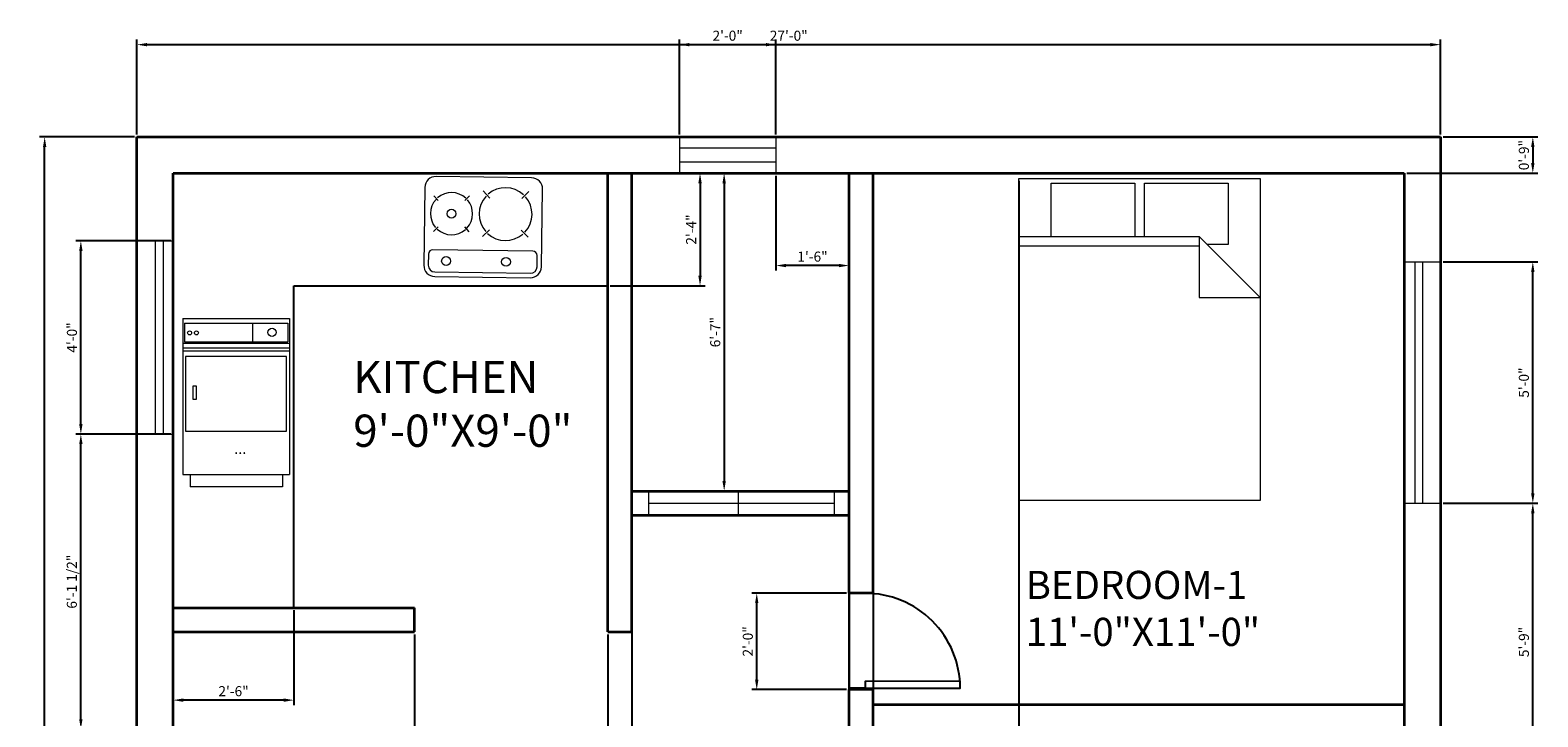
# Model space of a CAD drawing. Units: inches. Extents: x -2945 to -2182, y 3541 to 4172.
# Tile 5 of 5: x -2558 to -2183, y 3865 to 4036. Entities that reach past the tile are written whole.
import ezdxf
from ezdxf.enums import TextEntityAlignment as Align

# ---------------------------------------------------------------- set-up
doc = ezdxf.new("R2010")
doc.units = ezdxf.units.IN
for name, color, linetype, lineweight in [('A-ANNO-DIMS', 2, 'Continuous', 18), ('A-AREA-IDEN', 7, 'Continuous', 18), ('A-DOOR', 3, 'Continuous', 25), ('A-EQPM', 8, 'Continuous', 18), ('A-FLOR-FIXT', 9, 'Continuous', 25), ('A-FURN', 9, 'Continuous', 18), ('A-GLAZ', 4, 'Continuous', 18), ('A-WALL', 7, 'Continuous', 35)]:
    doc.layers.add(name, color=color, linetype=linetype, lineweight=lineweight)
doc.styles.add('OPUS', font='txt')
doc.styles.get("Standard").update_dxf_attribs({"font": 'arial.ttf'})
doc.dimstyles.new('ISO-25', dxfattribs={"dimtxt": 2.5, "dimasz": 2.5, "dimexe": 1.25, "dimexo": 0.625, "dimtad": 1, "dimdec": 0, "dimlunit": 3, "dimtxsty": 'Standard', "dimcen": 2.5, "dimadec": 0, "dimazin": 0, "dimtfac": 1, "dimtdec": 0, "dimtmove": 0, "dimatfit": 3, "dimfxl": 1, "dimarcsym": 0})

# ---------------------------------------------------------------- blocks, each defined once
blk = doc.blocks.new('Bed - Queen')
for p, q in [((0, -80.00003), (0, 0)), ((0, 0), (59.99999, 0)), ((59.99999, 0), (59.99999, -80.00003)), ((7.99999, -1.2), (28.79998, -1.2)), ((7.99999, -14.4), (7.99999, -1.2)), ((28.79998, -1.2), (28.79998, -14.4)), ((31.19999, -1.2), (51.99999, -1.2)), ((31.19999, -14.4), (31.19999, -1.2)), ((51.99999, -1.2), (51.99999, -16.4)), ((0, -14.4), (44.8, -14.4)), ((59.99999, -29.6), (44.8, -14.4)), ((44.8, -14.4), (44.8, -29.6)), ((44.8, -16.8), (0, -16.8)), ((51.99999, -16.4), (46.79936, -16.4)), ((44.8, -29.6), (59.99999, -29.6)), ((59.99999, -80.00003), (0, -80.00003))]:
    blk.add_line(p, q)
blk = doc.blocks.new('*U5')
for p, q in [((-600, 0), (-600, -100)), ((0, 0), (0, -100))]:
    blk.add_line(p, q)
blk.add_lwpolyline([(0, 0), (0, 600), (-43.75, 600), (-43.75, 0)], close=True)
blk.add_arc((0, 0), 600, 90, 180)
blk = doc.blocks.new('COOKTOP-2B')
for p, q in [((26.79, 24.83), (3.07, 25.16)), ((0.27, 22.44), (0, 3.13)), ((2.48, 20.39), (3.6, 19.22)), ((11.35, 20.32), (10.18, 19.2)), ((14.72, 21.57), (16.43, 19.81)), ((26.08, 21.42), (24.32, 19.71)), ((29.25, 2.72), (29.51, 22.03)), ((2.41, 11.52), (3.59, 12.64)), ((11.28, 11.45), (10.16, 12.63)), ((14.56, 10.21), (16.33, 11.92)), ((25.93, 10.06), (24.22, 11.82)), ((1.14, 5.87), (1.1, 3.11)), ((27.09, 6.61), (2.26, 6.96)), ((28.14, 2.74), (28.18, 5.5)), ((2.72, 0.33), (26.45, 0)), ((2.74, 1.43), (26.46, 1.1))]:
    blk.add_line(p, q)
for centre in [(6.88, 15.92), (5.53, 4.15), (20.43, 3.95)]:
    blk.add_circle(centre, 1.1)
for centre, radius, start, end in [((3.03, 22.4), 2.76, 89.203, 179.203), ((26.76, 22.07), 2.76, 359.203, 89.203), ((6.88, 15.92), 5.24, 137.22, 221.186), ((6.88, 15.92), 5.24, 47.22, 131.186), ((6.88, 15.92), 5.24, 317.22, 41.186), ((20.32, 15.81), 6.57, 137.22, 221.186), ((20.32, 15.81), 6.57, 47.22, 131.186), ((20.32, 15.81), 6.57, 317.22, 41.186), ((6.88, 15.92), 5.24, 227.22, 311.186), ((20.32, 15.81), 6.57, 227.22, 311.186), ((2.25, 5.86), 1.1, 89.203, 179.203), ((27.08, 5.51), 1.1, 359.203, 89.203), ((2.76, 3.09), 2.76, 179.203, 269.203), ((2.76, 3.09), 1.66, 179.203, 269.203), ((26.49, 2.76), 2.76, 269.203, 359.203), ((26.49, 2.76), 1.66, 269.203, 359.203)]:
    blk.add_arc(centre, radius, start, end)
blk = doc.blocks.new('KITCHEN-APPLIANCE-FRONT')
for p, q in [((0, 41.84), (0, 3.07)), ((0, 41.84), (26.49, 41.84)), ((26.49, 41.84), (26.49, 3.07)), ((0.38, 40.69), (0.38, 36.08)), ((0.38, 40.69), (26.1, 40.69)), ((17.27, 40.69), (17.27, 36.08)), ((26.1, 40.69), (26.1, 36.08)), ((0, 35.7), (26.49, 35.7)), ((0, 34.55), (26.49, 34.55)), ((0, 33.78), (26.49, 33.78)), ((0.38, 36.08), (26.1, 36.08)), ((0, 3.07), (26.49, 3.07)), ((1.77, 3.07), (1.77, 0)), ((24.72, 0), (1.77, 0)), ((24.72, 3.07), (24.72, 0))]:
    blk.add_line(p, q)
for points in [[(0.62, 13.82), (25.76, 13.82), (25.76, 32.44), (0.62, 32.44)], [(2.53, 21.69), (2.53, 25.14), (3.3, 25.14), (3.3, 21.69)]]:
    blk.add_lwpolyline(points, close=True)
for centre, radius in [((1.65, 38.28), 0.491), ((3.34, 38.28), 0.491), ((22.13, 38.4), 1.02)]:
    blk.add_circle(centre, radius)
at = {"style": 'OPUS'}
blk.add_text('...', height=2.65, dxfattribs=at).set_placement((14.24, 8.2), align=Align.CENTER)
blk = doc.blocks.new('*D20')
at = {"layer": 'A-ANNO-DIMS', "color": 0, "lineweight": -2, "transparency": 16777216}
for p, q in [((-2531.05, 4010.2), (-2531.05, 4033.78)), ((-2528.55, 4032.53), (-2209.55, 4032.53)), ((-2207.05, 4010.2), (-2207.05, 4033.78))]:
    blk.add_line(p, q, dxfattribs=at)
at = {"layer": 'A-ANNO-DIMS', "color": 0, "transparency": 16777216}
for points in [[(-2528.55, 4032.94), (-2528.55, 4032.11), (-2531.05, 4032.53)], [(-2209.55, 4032.94), (-2209.55, 4032.11), (-2207.05, 4032.53)]]:
    blk.add_solid(points, dxfattribs=at)
at = {"layer": 'Defpoints', "color": 0, "transparency": 16777216}
for p in [(-2207.05, 4032.53), (-2531.05, 4009.58), (-2207.05, 4009.58)]:
    blk.add_point(p, dxfattribs=at)
at = {"layer": 'A-ANNO-DIMS', "color": 0, "transparency": 16777216, "insert": (-2369.05, 4034.43), "char_height": 2.5, "attachment_point": 5}
blk.add_mtext('27\'-0"', dxfattribs=at)
blk = doc.blocks.new('*D21')
at = {"layer": 'A-ANNO-DIMS', "color": 0, "lineweight": -2, "transparency": 16777216}
for p, q in [((-2531.67, 4009.58), (-2555.25, 4009.58)), ((-2554, 3568.08), (-2554, 4007.08)), ((-2531.67, 3565.58), (-2555.25, 3565.58))]:
    blk.add_line(p, q, dxfattribs=at)
at = {"layer": 'A-ANNO-DIMS', "color": 0, "transparency": 16777216}
for points in [[(-2554.42, 4007.08), (-2553.58, 4007.08), (-2554, 4009.58)], [(-2554.42, 3568.08), (-2553.58, 3568.08), (-2554, 3565.58)]]:
    blk.add_solid(points, dxfattribs=at)
at = {"layer": 'Defpoints', "color": 0, "transparency": 16777216}
for p in [(-2554, 4009.58), (-2531.05, 4009.58), (-2531.05, 3565.58)]:
    blk.add_point(p, dxfattribs=at)
at = {"layer": 'A-ANNO-DIMS', "color": 0, "transparency": 16777216, "insert": (-2555.9, 3787.58), "char_height": 2.5, "attachment_point": 5, "rotation": 90}
blk.add_mtext('37\'-0"', dxfattribs=at)
blk = doc.blocks.new('*D29')
at = {"layer": 'A-ANNO-DIMS', "color": 0, "lineweight": -2, "transparency": 16777216}
for p, q in [((-2522.67, 3935.75), (-2546.25, 3935.75)), ((-2545, 3864.89), (-2545, 3933.25)), ((-2522.67, 3862.39), (-2546.25, 3862.39))]:
    blk.add_line(p, q, dxfattribs=at)
at = {"layer": 'A-ANNO-DIMS', "color": 0, "transparency": 16777216}
for points in [[(-2545.42, 3933.25), (-2544.58, 3933.25), (-2545, 3935.75)], [(-2545.42, 3864.89), (-2544.58, 3864.89), (-2545, 3862.39)]]:
    blk.add_solid(points, dxfattribs=at)
at = {"layer": 'Defpoints', "color": 0, "transparency": 16777216}
for p in [(-2545, 3935.75), (-2522.05, 3935.75), (-2522.05, 3862.39)]:
    blk.add_point(p, dxfattribs=at)
at = {"layer": 'A-ANNO-DIMS', "color": 0, "transparency": 16777216, "insert": (-2546.92, 3899.07), "char_height": 2.5, "attachment_point": 5, "rotation": 90}
blk.add_mtext('6\'-1 1/2"', dxfattribs=at)
blk = doc.blocks.new('*D30')
at = {"layer": 'A-ANNO-DIMS', "color": 0, "lineweight": -2, "transparency": 16777216}
for p, q in [((-2522.67, 3983.75), (-2546.25, 3983.75)), ((-2545, 3938.25), (-2545, 3981.25)), ((-2522.67, 3935.75), (-2546.25, 3935.75))]:
    blk.add_line(p, q, dxfattribs=at)
at = {"layer": 'A-ANNO-DIMS', "color": 0, "transparency": 16777216}
for points in [[(-2545.42, 3981.25), (-2544.58, 3981.25), (-2545, 3983.75)], [(-2545.42, 3938.25), (-2544.58, 3938.25), (-2545, 3935.75)]]:
    blk.add_solid(points, dxfattribs=at)
at = {"layer": 'Defpoints', "color": 0, "transparency": 16777216}
for p in [(-2545, 3983.75), (-2522.05, 3983.75), (-2522.05, 3935.75)]:
    blk.add_point(p, dxfattribs=at)
at = {"layer": 'A-ANNO-DIMS', "color": 0, "transparency": 16777216, "insert": (-2546.9, 3959.75), "char_height": 2.5, "attachment_point": 5, "rotation": 90}
blk.add_mtext('4\'-0"', dxfattribs=at)
blk = doc.blocks.new('*D31')
at = {"layer": 'A-ANNO-DIMS', "color": 0, "lineweight": -2, "transparency": 16777216}
for p, q in [((-2372.23, 3999.95), (-2372.23, 3976.38)), ((-2354.05, 3999.95), (-2354.05, 3976.38)), ((-2356.55, 3977.63), (-2369.73, 3977.63))]:
    blk.add_line(p, q, dxfattribs=at)
at = {"layer": 'A-ANNO-DIMS', "color": 0, "transparency": 16777216}
for points in [[(-2369.73, 3978.04), (-2369.73, 3977.21), (-2372.23, 3977.63)], [(-2356.55, 3978.04), (-2356.55, 3977.21), (-2354.05, 3977.63)]]:
    blk.add_solid(points, dxfattribs=at)
at = {"layer": 'Defpoints', "color": 0, "transparency": 16777216}
for p in [(-2372.23, 4000.58), (-2354.05, 4000.58), (-2372.23, 3977.63)]:
    blk.add_point(p, dxfattribs=at)
at = {"layer": 'A-ANNO-DIMS', "color": 0, "transparency": 16777216, "insert": (-2363.14, 3979.53), "char_height": 2.5, "attachment_point": 5}
blk.add_mtext('1\'-6"', dxfattribs=at)
blk = doc.blocks.new('*D32')
at = {"layer": 'A-ANNO-DIMS', "color": 0, "lineweight": -2, "transparency": 16777216}
for p, q in [((-2396.23, 4010.2), (-2396.23, 4033.78)), ((-2393.73, 4032.53), (-2374.73, 4032.53)), ((-2372.23, 4010.2), (-2372.23, 4033.78))]:
    blk.add_line(p, q, dxfattribs=at)
at = {"layer": 'A-ANNO-DIMS', "color": 0, "transparency": 16777216}
for points in [[(-2393.73, 4032.94), (-2393.73, 4032.11), (-2396.23, 4032.53)], [(-2374.73, 4032.94), (-2374.73, 4032.11), (-2372.23, 4032.53)]]:
    blk.add_solid(points, dxfattribs=at)
at = {"layer": 'Defpoints', "color": 0, "transparency": 16777216}
for p in [(-2372.23, 4032.53), (-2396.23, 4009.58), (-2372.23, 4009.58)]:
    blk.add_point(p, dxfattribs=at)
at = {"layer": 'A-ANNO-DIMS', "color": 0, "transparency": 16777216, "insert": (-2384.23, 4034.43), "char_height": 2.5, "attachment_point": 5}
blk.add_mtext('2\'-0"', dxfattribs=at)
blk = doc.blocks.new('*D39')
at = {"layer": 'A-ANNO-DIMS', "color": 0, "lineweight": -2, "transparency": 16777216}
for p, q in [((-2206.42, 3918.54), (-2182.85, 3918.54)), ((-2184.1, 3852.12), (-2184.1, 3916.04)), ((-2206.42, 3849.62), (-2182.85, 3849.62))]:
    blk.add_line(p, q, dxfattribs=at)
at = {"layer": 'A-ANNO-DIMS', "color": 0, "transparency": 16777216}
for points in [[(-2184.52, 3916.04), (-2183.68, 3916.04), (-2184.1, 3918.54)], [(-2184.52, 3852.12), (-2183.68, 3852.12), (-2184.1, 3849.62)]]:
    blk.add_solid(points, dxfattribs=at)
at = {"layer": 'Defpoints', "color": 0, "transparency": 16777216}
for p in [(-2207.05, 3918.54), (-2184.1, 3918.54), (-2207.05, 3849.62)]:
    blk.add_point(p, dxfattribs=at)
at = {"layer": 'A-ANNO-DIMS', "color": 0, "transparency": 16777216, "insert": (-2186, 3884.08), "char_height": 2.5, "attachment_point": 5, "rotation": 90}
blk.add_mtext('5\'-9"', dxfattribs=at)
blk = doc.blocks.new('*D40')
at = {"layer": 'A-ANNO-DIMS', "color": 0, "lineweight": -2, "transparency": 16777216}
for p, q in [((-2206.42, 3978.54), (-2182.85, 3978.54)), ((-2184.1, 3921.04), (-2184.1, 3976.04)), ((-2206.42, 3918.54), (-2182.85, 3918.54))]:
    blk.add_line(p, q, dxfattribs=at)
at = {"layer": 'A-ANNO-DIMS', "color": 0, "transparency": 16777216}
for points in [[(-2184.52, 3976.04), (-2183.68, 3976.04), (-2184.1, 3978.54)], [(-2184.52, 3921.04), (-2183.68, 3921.04), (-2184.1, 3918.54)]]:
    blk.add_solid(points, dxfattribs=at)
at = {"layer": 'Defpoints', "color": 0, "transparency": 16777216}
for p in [(-2207.05, 3978.54), (-2184.1, 3978.54), (-2207.05, 3918.54)]:
    blk.add_point(p, dxfattribs=at)
at = {"layer": 'A-ANNO-DIMS', "color": 0, "transparency": 16777216, "insert": (-2186, 3948.54), "char_height": 2.5, "attachment_point": 5, "rotation": 90}
blk.add_mtext('5\'-0"', dxfattribs=at)
blk = doc.blocks.new('*D41')
at = {"layer": 'A-ANNO-DIMS', "color": 0, "lineweight": -2, "transparency": 16777216}
for p, q in [((-2408.05, 3920.95), (-2408.05, 3541.38)), ((-2354.05, 3920.95), (-2354.05, 3541.38)), ((-2405.55, 3542.63), (-2356.55, 3542.63))]:
    blk.add_line(p, q, dxfattribs=at)
at = {"layer": 'A-ANNO-DIMS', "color": 0, "transparency": 16777216}
for points in [[(-2405.55, 3543.04), (-2405.55, 3542.21), (-2408.05, 3542.63)], [(-2356.55, 3543.04), (-2356.55, 3542.21), (-2354.05, 3542.63)]]:
    blk.add_solid(points, dxfattribs=at)
at = {"layer": 'Defpoints', "color": 0, "transparency": 16777216}
for p in [(-2408.05, 3921.58), (-2354.05, 3921.58), (-2354.05, 3542.63)]:
    blk.add_point(p, dxfattribs=at)
at = {"layer": 'A-ANNO-DIMS', "color": 0, "transparency": 16777216, "insert": (-2381.05, 3544.53), "char_height": 2.5, "attachment_point": 5}
blk.add_mtext('4\'-6"', dxfattribs=at)
blk = doc.blocks.new('*D42')
at = {"layer": 'A-ANNO-DIMS', "color": 0, "lineweight": -2, "transparency": 16777216}
for p, q in [((-2407.42, 4000.58), (-2383.85, 4000.58)), ((-2385.1, 3998.08), (-2385.1, 3924.08)), ((-2407.42, 3921.58), (-2383.85, 3921.58))]:
    blk.add_line(p, q, dxfattribs=at)
at = {"layer": 'A-ANNO-DIMS', "color": 0, "transparency": 16777216}
for points in [[(-2385.52, 3998.08), (-2384.68, 3998.08), (-2385.1, 4000.58)], [(-2385.52, 3924.08), (-2384.68, 3924.08), (-2385.1, 3921.58)]]:
    blk.add_solid(points, dxfattribs=at)
at = {"layer": 'Defpoints', "color": 0, "transparency": 16777216}
for p in [(-2408.05, 4000.58), (-2408.05, 3921.58), (-2385.1, 3921.58)]:
    blk.add_point(p, dxfattribs=at)
at = {"layer": 'A-ANNO-DIMS', "color": 0, "transparency": 16777216, "insert": (-2387, 3961.08), "char_height": 2.5, "attachment_point": 5, "rotation": 90}
blk.add_mtext('6\'-7"', dxfattribs=at)
blk = doc.blocks.new('*D43')
at = {"layer": 'A-ANNO-DIMS', "color": 0, "lineweight": -2, "transparency": 16777216}
for p, q in [((-2522.05, 3891.95), (-2522.05, 3868.38)), ((-2492.05, 3891.95), (-2492.05, 3868.38)), ((-2494.55, 3869.63), (-2519.55, 3869.63))]:
    blk.add_line(p, q, dxfattribs=at)
at = {"layer": 'A-ANNO-DIMS', "color": 0, "transparency": 16777216}
for points in [[(-2519.55, 3870.04), (-2519.55, 3869.21), (-2522.05, 3869.63)], [(-2494.55, 3870.04), (-2494.55, 3869.21), (-2492.05, 3869.63)]]:
    blk.add_solid(points, dxfattribs=at)
at = {"layer": 'Defpoints', "color": 0, "transparency": 16777216}
for p in [(-2522.05, 3892.58), (-2492.05, 3892.58), (-2522.05, 3869.63)]:
    blk.add_point(p, dxfattribs=at)
at = {"layer": 'A-ANNO-DIMS', "color": 0, "transparency": 16777216, "insert": (-2507.05, 3871.53), "char_height": 2.5, "attachment_point": 5}
blk.add_mtext('2\'-6"', dxfattribs=at)
blk = doc.blocks.new('*D44')
at = {"layer": 'A-ANNO-DIMS', "color": 0, "lineweight": -2, "transparency": 16777216}
for p, q in [((-2413.42, 4000.58), (-2389.85, 4000.58)), ((-2391.1, 3998.08), (-2391.1, 3975.08)), ((-2413.42, 3972.58), (-2389.85, 3972.58))]:
    blk.add_line(p, q, dxfattribs=at)
at = {"layer": 'A-ANNO-DIMS', "color": 0, "transparency": 16777216}
for points in [[(-2391.52, 3998.08), (-2390.68, 3998.08), (-2391.1, 4000.58)], [(-2391.52, 3975.08), (-2390.68, 3975.08), (-2391.1, 3972.58)]]:
    blk.add_solid(points, dxfattribs=at)
at = {"layer": 'Defpoints', "color": 0, "transparency": 16777216}
for p in [(-2414.05, 4000.58), (-2414.05, 3972.58), (-2391.1, 3972.58)]:
    blk.add_point(p, dxfattribs=at)
at = {"layer": 'A-ANNO-DIMS', "color": 0, "transparency": 16777216, "insert": (-2392.98, 3986.58), "char_height": 2.5, "attachment_point": 5, "rotation": 90}
blk.add_mtext('2\'-4"', dxfattribs=at)
blk = doc.blocks.new('*D45')
at = {"layer": 'A-ANNO-DIMS', "color": 0, "lineweight": -2, "transparency": 16777216}
for p, q in [((-2414.05, 3885.95), (-2414.05, 3541.38)), ((-2408.05, 3885.95), (-2408.05, 3541.38)), ((-2416.55, 3542.63), (-2419.05, 3542.63)), ((-2414.05, 3542.63), (-2408.05, 3542.63)), ((-2405.55, 3542.63), (-2395.15, 3542.63))]:
    blk.add_line(p, q, dxfattribs=at)
at = {"layer": 'A-ANNO-DIMS', "color": 0, "transparency": 16777216}
for points in [[(-2416.55, 3543.04), (-2416.55, 3542.21), (-2414.05, 3542.63)], [(-2405.55, 3543.04), (-2405.55, 3542.21), (-2408.05, 3542.63)]]:
    blk.add_solid(points, dxfattribs=at)
at = {"layer": 'Defpoints', "color": 0, "transparency": 16777216}
for p in [(-2414.05, 3886.58), (-2408.05, 3886.58), (-2408.05, 3542.63)]:
    blk.add_point(p, dxfattribs=at)
at = {"layer": 'A-ANNO-DIMS', "color": 0, "transparency": 16777216, "insert": (-2399.1, 3544.53), "char_height": 2.5, "attachment_point": 5}
blk.add_mtext('0\'-6"', dxfattribs=at)
blk = doc.blocks.new('*D46')
at = {"layer": 'A-ANNO-DIMS', "color": 0, "lineweight": -2, "transparency": 16777216}
for p, q in [((-2206.42, 4009.58), (-2182.85, 4009.58)), ((-2184.1, 4007.08), (-2184.1, 4003.08)), ((-2215.42, 4000.58), (-2182.85, 4000.58))]:
    blk.add_line(p, q, dxfattribs=at)
at = {"layer": 'A-ANNO-DIMS', "color": 0, "transparency": 16777216}
for points in [[(-2184.52, 4007.08), (-2183.68, 4007.08), (-2184.1, 4009.58)], [(-2184.52, 4003.08), (-2183.68, 4003.08), (-2184.1, 4000.58)]]:
    blk.add_solid(points, dxfattribs=at)
at = {"layer": 'Defpoints', "color": 0, "transparency": 16777216}
for p in [(-2207.05, 4009.58), (-2216.05, 4000.58), (-2184.1, 4000.58)]:
    blk.add_point(p, dxfattribs=at)
at = {"layer": 'A-ANNO-DIMS', "color": 0, "transparency": 16777216, "insert": (-2186, 4005.08), "char_height": 2.5, "attachment_point": 5, "rotation": 90}
blk.add_mtext('0\'-9"', dxfattribs=at)
blk = doc.blocks.new('*D47')
at = {"layer": 'A-ANNO-DIMS', "color": 0, "lineweight": -2, "transparency": 16777216}
for p, q in [((-2462.05, 3885.95), (-2462.05, 3541.38)), ((-2414.05, 3885.95), (-2414.05, 3541.38)), ((-2459.55, 3542.63), (-2416.55, 3542.63))]:
    blk.add_line(p, q, dxfattribs=at)
at = {"layer": 'A-ANNO-DIMS', "color": 0, "transparency": 16777216}
for points in [[(-2459.55, 3543.04), (-2459.55, 3542.21), (-2462.05, 3542.63)], [(-2416.55, 3543.04), (-2416.55, 3542.21), (-2414.05, 3542.63)]]:
    blk.add_solid(points, dxfattribs=at)
at = {"layer": 'Defpoints', "color": 0, "transparency": 16777216}
for p in [(-2462.05, 3886.58), (-2414.05, 3886.58), (-2414.05, 3542.63)]:
    blk.add_point(p, dxfattribs=at)
at = {"layer": 'A-ANNO-DIMS', "color": 0, "transparency": 16777216, "insert": (-2438.05, 3544.53), "char_height": 2.5, "attachment_point": 5}
blk.add_mtext('4\'-0"', dxfattribs=at)
blk = doc.blocks.new('*D49')
at = {"layer": 'A-ANNO-DIMS', "color": 0, "lineweight": -2, "transparency": 16777216}
for p, q in [((-2354.67, 3896.23), (-2378.25, 3896.23)), ((-2377, 3874.73), (-2377, 3893.73)), ((-2354.67, 3872.23), (-2378.25, 3872.23))]:
    blk.add_line(p, q, dxfattribs=at)
at = {"layer": 'A-ANNO-DIMS', "color": 0, "transparency": 16777216}
for points in [[(-2377.42, 3893.73), (-2376.58, 3893.73), (-2377, 3896.23)], [(-2377.42, 3874.73), (-2376.58, 3874.73), (-2377, 3872.23)]]:
    blk.add_solid(points, dxfattribs=at)
at = {"layer": 'Defpoints', "color": 0, "transparency": 16777216}
for p in [(-2377, 3896.23), (-2354.05, 3896.23), (-2354.05, 3872.23)]:
    blk.add_point(p, dxfattribs=at)
at = {"layer": 'A-ANNO-DIMS', "color": 0, "transparency": 16777216, "insert": (-2378.9, 3884.23), "char_height": 2.5, "attachment_point": 5, "rotation": 90}
blk.add_mtext('2\'-0"', dxfattribs=at)
blk = doc.blocks.new('*D55')
at = {"layer": 'A-ANNO-DIMS', "color": 0, "lineweight": -2, "transparency": 16777216}
for p, q in [((-2348.05, 3999.95), (-2348.05, 3541.38)), ((-2311.84, 3998.65), (-2311.84, 3541.38)), ((-2345.55, 3542.63), (-2314.34, 3542.63))]:
    blk.add_line(p, q, dxfattribs=at)
at = {"layer": 'A-ANNO-DIMS', "color": 0, "transparency": 16777216}
for points in [[(-2345.55, 3543.04), (-2345.55, 3542.21), (-2348.05, 3542.63)], [(-2314.34, 3543.04), (-2314.34, 3542.21), (-2311.84, 3542.63)]]:
    blk.add_solid(points, dxfattribs=at)
at = {"layer": 'Defpoints', "color": 0, "transparency": 16777216}
for p in [(-2348.05, 4000.58), (-2311.84, 3999.28), (-2311.84, 3542.63)]:
    blk.add_point(p, dxfattribs=at)
at = {"layer": 'A-ANNO-DIMS', "color": 0, "transparency": 16777216, "insert": (-2329.94, 3544.53), "char_height": 2.5, "attachment_point": 5}
blk.add_mtext('3\'-0"', dxfattribs=at)

msp = doc.modelspace()

# ---------------------------------------------------------------- linework, layer by layer
at = {"layer": 'A-DOOR'}
msp.add_line((-2354.05, 3872.23), (-2354.05, 3896.23), dxfattribs=at)
at = {"layer": 'A-FLOR-FIXT'}
for p, q in [((-2492.05, 3892.58), (-2492.05, 3972.58)), ((-2492.05, 3972.58), (-2414.05, 3972.58))]:
    msp.add_line(p, q, dxfattribs=at)
at = {"layer": 'A-GLAZ'}
for p, q in [((-2396.23, 4009.58), (-2396.23, 4000.58)), ((-2396.23, 4006.85), (-2372.23, 4006.85)), ((-2372.23, 4009.58), (-2372.23, 4000.58)), ((-2396.23, 4003.39), (-2372.23, 4003.39)), ((-2531.05, 3983.75), (-2522.05, 3983.75)), ((-2526.55, 3983.75), (-2526.55, 3935.75)), ((-2524.54, 3983.75), (-2524.54, 3935.75)), ((-2216.05, 3978.54), (-2207.05, 3978.54)), ((-2213.43, 3978.54), (-2213.43, 3918.54)), ((-2211.55, 3978.54), (-2211.55, 3918.54)), ((-2531.05, 3935.75), (-2522.05, 3935.75)), ((-2403.88, 3921.61), (-2403.88, 3915.59)), ((-2381.62, 3921.61), (-2381.62, 3915.59)), ((-2357.75, 3921.61), (-2357.75, 3915.59)), ((-2403.88, 3918.6), (-2381.62, 3918.6)), ((-2381.62, 3918.6), (-2357.75, 3918.6)), ((-2216.05, 3918.54), (-2207.05, 3918.54))]:
    msp.add_line(p, q, dxfattribs=at)
at = {"layer": 'A-WALL'}
for p, q in [((-2531.05, 4009.58), (-2207.05, 4009.58)), ((-2531.05, 3565.58), (-2531.05, 4009.58)), ((-2207.05, 4009.58), (-2207.05, 3565.58)), ((-2522.05, 4000.58), (-2216.05, 4000.58)), ((-2522.05, 3574.58), (-2522.05, 4000.58)), ((-2414.05, 3886.58), (-2414.05, 4000.58)), ((-2408.05, 3886.58), (-2408.05, 4000.58)), ((-2354.05, 3896.23), (-2354.05, 4000.58)), ((-2348.05, 3896.23), (-2348.05, 4000.58)), ((-2216.05, 4000.58), (-2216.05, 3574.58)), ((-2408.05, 3921.58), (-2354.05, 3921.58)), ((-2408.05, 3915.58), (-2354.05, 3915.58)), ((-2348.05, 3896.23), (-2354.05, 3896.23)), ((-2522.05, 3892.58), (-2462.05, 3892.58)), ((-2462.05, 3886.58), (-2462.05, 3892.58)), ((-2522.05, 3886.58), (-2462.05, 3886.58)), ((-2414.05, 3886.58), (-2408.05, 3886.58)), ((-2348.05, 3872.23), (-2354.05, 3872.23)), ((-2354.05, 3860.25), (-2354.05, 3872.23)), ((-2348.05, 3860.25), (-2348.05, 3872.23)), ((-2348.05, 3868.58), (-2216.05, 3868.58))]:
    msp.add_line(p, q, dxfattribs=at)

# ---------------------------------------------------------------- block references
at = {"layer": 'A-DOOR', "xscale": 0.0393700787401575, "yscale": 0.0393700787401575, "zscale": 0.0393700787401575, "rotation": 270.1211645851394}
msp.add_blockref('*U5', (-2350.05, 3872.57), dxfattribs=at)
at = {"layer": 'A-EQPM'}
for name, p in [('COOKTOP-2B', (-2459.75, 3974.6)), ('KITCHEN-APPLIANCE-FRONT', (-2519.62, 3922.62))]:
    msp.add_blockref(name, p, dxfattribs=at)
at = {"layer": 'A-FURN'}
msp.add_blockref('Bed - Queen', (-2311.84, 3999.28), dxfattribs=at)

# ---------------------------------------------------------------- texts
at = {"layer": 'A-AREA-IDEN', "attachment_point": 1}
for s, width, heights, insert, char_height in [('KITCHEN\\P9\'-0"X9\'-0"', 51.4369, [29.22], (-2477.29, 3953.92), 8), ('BEDROOM-1\\P11\'-0"X11\'-0"', 36.5253, [0], (-2310.15, 3901.76), 7)]:
    msp.add_mtext_dynamic_manual_height_columns(s, width=width, gutter_width=12.5, heights=heights, dxfattribs=dict(at, insert=insert, char_height=char_height))

# ---------------------------------------------------------------- dimensions: what is measured, and where the dimension line sits
at = {"layer": 'A-ANNO-DIMS'}
for base, p1, p2, picture, middle in [((-2207.05, 4032.53), (-2531.05, 4009.58), (-2207.05, 4009.58), '*D20', (-2369.05, 4034.43)), ((-2372.23, 4032.53), (-2396.23, 4009.58), (-2372.23, 4009.58), '*D32', (-2384.23, 4034.43)), ((-2311.84, 3542.63), (-2348.05, 4000.58), (-2311.84, 3999.28), '*D55', (-2329.94, 3544.53)), ((-2354.05, 3542.63), (-2408.05, 3921.58), (-2354.05, 3921.58), '*D41', (-2381.05, 3544.53)), ((-2414.05, 3542.63), (-2462.05, 3886.58), (-2414.05, 3886.58), '*D47', (-2438.05, 3544.53)), ((-2408.05, 3542.63), (-2414.05, 3886.58), (-2408.05, 3886.58), '*D45', (-2399.1, 3544.53))]:
    dim = msp.add_linear_dim(base=base, p1=p1, p2=p2, dimstyle='ISO-25', override={"dimdec": 1, "dimlfac": 1, "dimrnd": 0, "dimzin": 1, "dimdsep": 46, "dimlunit": 4, "dimfrac": 2}, dxfattribs=at)
    dim.commit()
    dim.dimension.update_dxf_attribs({"geometry": picture, "text_midpoint": middle})
for base, p1, p2, angle, picture, middle in [((-2554, 4009.58), (-2531.05, 3565.58), (-2531.05, 4009.58), 90, '*D21', (-2555.9, 3787.58)), ((-2184.1, 4000.58), (-2207.05, 4009.58), (-2216.05, 4000.58), 90, '*D46', (-2186, 4005.08)), ((-2391.1, 3972.58), (-2414.05, 4000.58), (-2414.05, 3972.58), 270, '*D44', (-2392.98, 3986.58)), ((-2385.1, 3921.58), (-2408.05, 4000.58), (-2408.05, 3921.58), 270, '*D42', (-2387, 3961.08)), ((-2372.23, 3977.63), (-2354.05, 4000.58), (-2372.23, 4000.58), 180, '*D31', (-2363.14, 3979.53)), ((-2545, 3983.75), (-2522.05, 3935.75), (-2522.05, 3983.75), 90, '*D30', (-2546.9, 3959.75)), ((-2184.1, 3978.54), (-2207.05, 3918.54), (-2207.05, 3978.54), 90, '*D40', (-2186, 3948.54)), ((-2545, 3935.75), (-2522.05, 3862.39), (-2522.05, 3935.75), 90, '*D29', (-2546.92, 3899.07)), ((-2184.1, 3918.54), (-2207.05, 3849.62), (-2207.05, 3918.54), 90, '*D39', (-2186, 3884.08)), ((-2377, 3896.23), (-2354.05, 3872.23), (-2354.05, 3896.23), 90, '*D49', (-2378.9, 3884.23)), ((-2522.05, 3869.63), (-2492.05, 3892.58), (-2522.05, 3892.58), 180, '*D43', (-2507.05, 3871.53))]:
    dim = msp.add_linear_dim(base=base, p1=p1, p2=p2, angle=angle, dimstyle='ISO-25', override={"dimdec": 1, "dimlfac": 1, "dimrnd": 0, "dimzin": 1, "dimdsep": 46, "dimlunit": 4, "dimfrac": 2}, dxfattribs=at)
    dim.commit()
    dim.dimension.update_dxf_attribs({"geometry": picture, "text_midpoint": middle})

doc.saveas('drawing.dxf')
